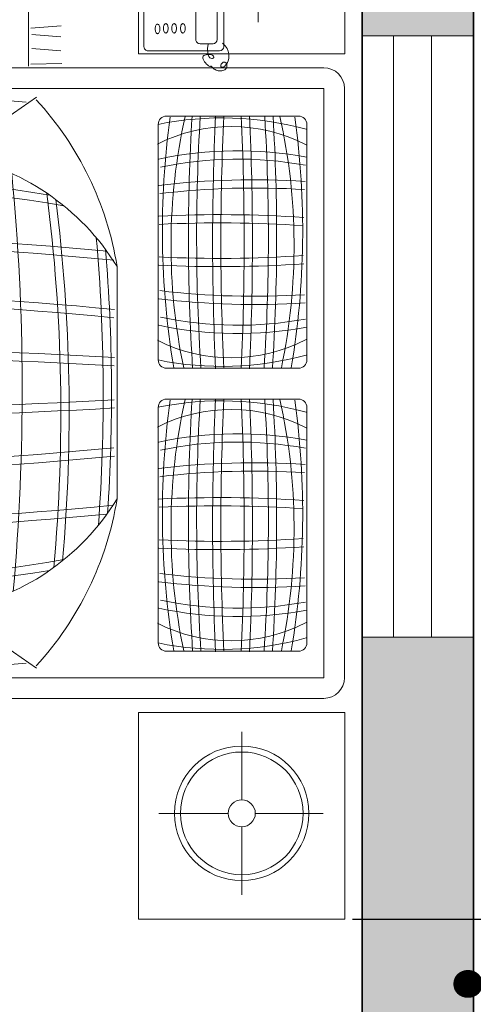
# Model space of a CAD drawing. Units: inches. Extents: x 1763 to 2368, y 1500 to 2097.
# Tile 20 of 24: x 2152 to 2189, y 1856 to 1935. Entities that reach past the tile are written whole.
import ezdxf

# ---------------------------------------------------------------- set-up
doc = ezdxf.new("R2010")
doc.units = ezdxf.units.IN
for name, color, linetype, lineweight in [('A-ANNO-DIMS', 2, 'Continuous', 18), ('A-FURN', 8, 'Continuous', 18), ('A-WALL', 7, 'Continuous', 35), ('A-WALL-PATT', 7, 'Continuous', 13), ('windows', 1, 'Continuous', 18)]:
    doc.layers.add(name, color=color, linetype=linetype, lineweight=lineweight)
doc.styles.get("Standard").update_dxf_attribs({"font": 'arial.ttf'})
doc.dimstyles.new('ISO-25', dxfattribs={"dimtxt": 12.5, "dimasz": 2.5, "dimexe": 1.25, "dimexo": 0.625, "dimtad": 1, "dimdec": 0, "dimlunit": 4, "dimtxsty": 'Standard', "dimblk": 'ARCHTICK', "dimcen": 2.5, "dimclrd": 3, "dimclrt": 4, "dimadec": 0, "dimazin": 0, "dimtfac": 1, "dimtdec": 0, "dimtmove": 0, "dimatfit": 3, "dimfxl": 1, "dimarcsym": 0})

# ---------------------------------------------------------------- blocks, each defined once
blk = doc.blocks.new('A$C77DF40FE')
for p, q in [((0.5, 2.6723), (0, 2.6723)), ((0.5, 2.1723), (0.5, 2.6723)), ((0.5839, 2.6714), (2.0097, 2.6714)), ((2.0936, 2.1723), (2.0936, 2.6723)), ((2.0936, 2.6723), (2.5936, 2.6723)), ((2.5936, 2.6723), (2.5936, 2.1723)), ((0.5339, 0.6344), (0.5339, 2.6214)), ((0.5839, 2.6214), (2.0097, 2.6214)), ((0.5839, 0.6344), (0.5839, 2.6214)), ((2.0097, 2.6214), (2.0097, 0.6344)), ((2.0597, 2.6214), (2.0597, 0.6344)), ((2.3379, 2.4554), (2.3379, 2.6199)), ((1.2408, 2.5803), (0.6708, 2.5803)), ((1.9255, 2.5803), (1.3555, 2.5803)), ((0.6508, 2.5603), (0.6508, 2.2403)), ((1.2608, 2.2403), (1.2608, 2.5603)), ((1.3355, 2.5603), (1.3355, 2.2403)), ((1.9455, 2.2403), (1.9455, 2.5603)), ((0.2588, 2.4621), (0.4233, 2.4621)), ((2.3051, 2.4226), (2.1406, 2.4226)), ((2.5352, 2.4226), (2.3707, 2.4226)), ((0.4873, 2.387), (0.4809, 2.3823)), ((0.4937, 2.3899), (0.4873, 2.387)), ((0.5, 2.3914), (0.4937, 2.3899)), ((0.506, 2.3917), (0.5, 2.3914)), ((0.5117, 2.391), (0.506, 2.3917)), ((0.5168, 2.3897), (0.5117, 2.391)), ((0.5212, 2.3878), (0.5168, 2.3897)), ((0.521, 2.3828), (0.5205, 2.3816)), ((0.5219, 2.3839), (0.521, 2.3828)), ((0.5248, 2.3858), (0.5212, 2.3878)), ((0.523, 2.3849), (0.5219, 2.3839)), ((0.5244, 2.3856), (0.523, 2.3849)), ((0.5261, 2.3861), (0.5244, 2.3856)), ((0.5277, 2.3836), (0.5248, 2.3858)), ((0.5279, 2.3864), (0.5261, 2.3861)), ((0.5298, 2.3813), (0.5277, 2.3836)), ((0.5298, 2.3864), (0.5279, 2.3864)), ((0.5318, 2.3861), (0.5298, 2.3864)), ((0.5338, 2.3855), (0.5318, 2.3861)), ((0.5356, 2.3846), (0.5338, 2.3855)), ((0.5373, 2.3832), (0.5356, 2.3846)), ((0.5387, 2.3815), (0.5373, 2.3832)), ((2.3379, 2.2215), (2.3379, 2.3898)), ((0.4828, 2.3788, 10.4), (0.2438, 2.3788, 10.4)), ((0.4656, 2.363, 10.4), (0.2638, 2.363, 10.4)), ((0.4809, 2.3823), (0.4746, 2.3757)), ((0.4928, 2.1957, 10.4), (0.4928, 2.3688, 10.4)), ((0.5205, 2.3816), (0.5202, 2.3804)), ((0.5202, 2.3804), (0.5202, 2.379)), ((0.5202, 2.379), (0.5206, 2.3777)), ((0.5206, 2.3777), (0.5213, 2.3764)), ((0.5213, 2.3764), (0.5224, 2.3752)), ((0.5224, 2.3752), (0.5237, 2.374)), ((0.5237, 2.374), (0.5252, 2.3731)), ((0.5252, 2.3731), (0.5268, 2.3723)), ((0.5268, 2.3723), (0.5283, 2.3719)), ((0.5283, 2.3719), (0.5297, 2.3717)), ((0.5297, 2.3717), (0.531, 2.372)), ((0.5313, 2.3792), (0.5298, 2.3813)), ((0.531, 2.372), (0.5319, 2.3726)), ((0.5322, 2.3771), (0.5313, 2.3792)), ((0.5319, 2.3726), (0.5325, 2.3738)), ((0.5326, 2.3753), (0.5322, 2.3771)), ((0.5325, 2.3738), (0.5326, 2.3753)), ((0.5383, 2.3581), (0.5394, 2.3604)), ((0.5399, 2.3794), (0.5387, 2.3815)), ((0.5394, 2.3604), (0.5403, 2.3629)), ((0.5407, 2.377), (0.5399, 2.3794)), ((0.5403, 2.3629), (0.5409, 2.3657)), ((0.5412, 2.3743), (0.5407, 2.377)), ((0.5409, 2.3657), (0.5413, 2.3686)), ((0.5414, 2.3715), (0.5412, 2.3743)), ((0.5413, 2.3686), (0.5414, 2.3715)), ((0.4756, 2.3215, 10.4), (0.4756, 2.353, 10.4)), ((0.4767, 2.3409), (0.4876, 2.34)), ((0.4876, 2.34), (0.4961, 2.3402)), ((0.4961, 2.3402), (0.5023, 2.3413)), ((0.502, 2.3463), (0.5017, 2.3431)), ((0.5017, 2.3431), (0.5018, 2.3398)), ((0.5018, 2.3398), (0.5023, 2.3365)), ((0.5026, 2.3491), (0.502, 2.3463)), ((0.5023, 2.3413), (0.5067, 2.3431)), ((0.5023, 2.3365), (0.5031, 2.3334)), ((0.5035, 2.3514), (0.5026, 2.3491)), ((0.5047, 2.3531), (0.5035, 2.3514)), ((0.5059, 2.3542), (0.5047, 2.3531)), ((0.5073, 2.3548), (0.5059, 2.3542)), ((0.5067, 2.3431), (0.5095, 2.3452)), ((0.5086, 2.3549), (0.5073, 2.3548)), ((0.5097, 2.3544), (0.5086, 2.3549)), ((0.5095, 2.3452), (0.511, 2.3475)), ((0.5107, 2.3534), (0.5097, 2.3544)), ((0.5113, 2.3518), (0.5107, 2.3534)), ((0.511, 2.3475), (0.5115, 2.3498)), ((0.5115, 2.3498), (0.5113, 2.3518)), ((0.5193, 2.3325), (0.5222, 2.3349)), ((0.5222, 2.3349), (0.5249, 2.3374)), ((0.5249, 2.3374), (0.5271, 2.3398)), ((0.5271, 2.3398), (0.5288, 2.3419)), ((0.5288, 2.3419), (0.5299, 2.3436)), ((0.5299, 2.3436), (0.5305, 2.3449)), ((0.53, 2.3482), (0.5302, 2.3488)), ((0.5301, 2.3477), (0.53, 2.3482)), ((0.5303, 2.3472), (0.5301, 2.3477)), ((0.5302, 2.3488), (0.5308, 2.3495)), ((0.5306, 2.3466), (0.5303, 2.3472)), ((0.5305, 2.3449), (0.5307, 2.3459)), ((0.5307, 2.3459), (0.5306, 2.3466)), ((0.5308, 2.3495), (0.5317, 2.3504)), ((0.5317, 2.3504), (0.5329, 2.3515)), ((0.5329, 2.3515), (0.5342, 2.3528)), ((0.5342, 2.3528), (0.5356, 2.3543)), ((0.5356, 2.3543), (0.537, 2.3561)), ((0.537, 2.3561), (0.5383, 2.3581)), ((0.2638, 2.3115, 10.4), (0.4656, 2.3115, 10.4)), ((0.5031, 2.3334), (0.5043, 2.3309)), ((0.5043, 2.3309), (0.506, 2.329)), ((0.506, 2.329), (0.5081, 2.328)), ((0.5081, 2.328), (0.5106, 2.328)), ((0.5106, 2.328), (0.5134, 2.3288)), ((0.5134, 2.3288), (0.5163, 2.3304)), ((0.5163, 2.3304), (0.5193, 2.3325)), ((0.6708, 2.2203), (1.2408, 2.2203)), ((1.3555, 2.2203), (1.9255, 2.2203)), ((0, 2.1723), (0.5, 2.1723)), ((0.2438, 2.1857, 10.4), (0.4828, 2.1857, 10.4)), ((2.5936, 2.1723), (2.0936, 2.1723)), ((1.5773, 2.1205), (1.0147, 2.1205)), ((0.438, 1.9118), (0.4323, 1.9849)), ((0.4531, 1.9138), (0.4588, 1.9847)), ((0.4873, 1.9138), (0.493, 1.9847)), ((0.5249, 1.9118), (0.5233, 1.9865)), ((0.6051, 1.925), (0.7457, 1.7234)), ((1.9869, 1.925), (1.8463, 1.7234)), ((0.5301, 1.9057), (0.3112, 1.9057))]:
    blk.add_line(p, q)
for radius in [0.1629, 0.1484, 0.0328]:
    blk.add_circle((2.3379, 2.4226), radius)
for centre, radius, start, end in [((0.5839, 2.6214), 0.05, 90, 180), ((2.0097, 2.6214), 0.05, 0, 90), ((0.6708, 2.5603), 0.02, 90, 180), ((1.4247, 2.3742), 0.7696, 164.6112, 191.5679), ((1.0701, 2.3966), 0.3942, 152.5365, 206.92), ((1.6628, 2.4129), 0.928, 169.6087, 191.899), ((1.6628, 2.4129), 0.908, 169.6087, 191.899), ((2.7571, 2.4533), 1.9523, 176.3947, 186.8195), ((2.7571, 2.4533), 1.9323, 176.3947, 186.8195), ((-0.8455, 2.4533), 1.9323, 353.1805, 3.6053), ((-0.8455, 2.4533), 1.9523, 353.1805, 3.6053), ((0.2489, 2.4129), 0.908, 348.101, 10.3913), ((0.2489, 2.4129), 0.928, 348.101, 10.3913), ((0.8416, 2.3966), 0.3942, 333.08, 27.4635), ((0.4869, 2.3742), 0.7696, 348.4321, 15.3888), ((1.2408, 2.5603), 0.02, 0, 90), ((1.3555, 2.5603), 0.02, 90, 180), ((2.1094, 2.3742), 0.7696, 164.6112, 191.5679), ((1.7548, 2.3966), 0.3942, 152.5365, 206.92), ((2.3475, 2.4129), 0.928, 169.6087, 191.899), ((2.3475, 2.4129), 0.908, 169.6087, 191.899), ((3.4419, 2.4533), 1.9523, 176.3947, 186.8195), ((3.4419, 2.4533), 1.9323, 176.3947, 186.8195), ((-0.1608, 2.4533), 1.9323, 353.1805, 3.6053), ((-0.1608, 2.4533), 1.9523, 353.1805, 3.6053), ((0.9336, 2.4129), 0.908, 348.101, 10.3913), ((0.9336, 2.4129), 0.928, 348.101, 10.3913), ((1.5263, 2.3966), 0.3942, 333.08, 27.4635), ((1.1716, 2.3742), 0.7696, 348.4321, 15.3888), ((1.9255, 2.5603), 0.02, 0, 90), ((0.9635, 1.1066), 1.4427, 78.1527, 102.4906), ((0.9287, 0.5819), 1.9884, 80.4201, 97.9672), ((3.9259, 2.3685), 3.0367, 176.1432, 182.775), ((3.9259, 2.3685), 3.0167, 176.1432, 182.775), ((-2.0216, 2.3685), 3.0167, 357.225, 3.8568), ((-2.0216, 2.3685), 3.0367, 357.225, 3.8568), ((1.6482, 1.1066), 1.4427, 78.1527, 102.4906), ((1.6135, 0.5819), 1.9884, 80.4201, 97.9672), ((4.6106, 2.3685), 3.0367, 176.1432, 182.775), ((4.6106, 2.3685), 3.0167, 176.1432, 182.775), ((-1.3369, 2.3685), 3.0167, 357.225, 3.8568), ((-1.3369, 2.3685), 3.0367, 357.225, 3.8568), ((0.9445, -2.3575), 4.8647, 86.2671, 93.4563), ((1.6292, -2.3575), 4.8647, 86.2671, 93.4563), ((0.9445, -2.3575), 4.8447, 86.2671, 93.4563), ((1.6292, -2.3575), 4.8447, 86.2671, 93.4563), ((0.9561, -3.928), 6.3765, 87.24779, 92.75221), ((1.6408, -3.928), 6.3765, 87.24779, 92.75221), ((0.9561, -3.928), 6.3565, 87.24779, 92.75221), ((1.6408, -3.928), 6.3565, 87.24779, 92.75221), ((0.4656, 2.353, 10.4), 0.01, 0, 90), ((0.4828, 2.3688, 10.4), 0.01, 0, 90), ((0.9561, 8.7285), 6.3765, 267.24779, 272.75221), ((0.9561, 8.7285), 6.3565, 267.24779, 272.75221), ((1.6408, 8.7285), 6.3765, 267.24779, 272.75221), ((1.6408, 8.7285), 6.3565, 267.24779, 272.75221), ((0.4656, 2.3215, 10.4), 0.01, 270, 0), ((0.9445, 7.158), 4.8447, 266.5437, 273.7329), ((1.6292, 7.158), 4.8447, 266.5437, 273.7329), ((0.9445, 7.158), 4.8647, 266.5437, 273.7329), ((1.6292, 7.158), 4.8647, 266.5437, 273.7329), ((0.43, 2.2801, 10.4), 0.00304, 140.3607, 180), ((0.43, 2.2801, 10.4), 0.00304, 180, 219.6393), ((0.434, 2.2768, 10.4), 0.00822, 116.5651, 140.3607), ((0.434, 2.2834, 10.4), 0.00822, 219.6393, 243.4349), ((0.4367, 2.2714, 10.4), 0.0142, 101.7009, 116.5651), ((0.4367, 2.2887, 10.4), 0.0142, 243.4349, 258.2991), ((0.4367, 2.25, 10.4), 0.0142, 101.7009, 116.5651), ((0.4384, 2.263, 10.4), 0.0228, 90, 101.7009), ((0.4384, 2.2972, 10.4), 0.0228, 258.2991, 270), ((0.4384, 2.2415, 10.4), 0.0228, 90, 101.7009), ((0.4384, 2.263, 10.4), 0.0228, 78.2991, 90), ((0.4384, 2.2972, 10.4), 0.0228, 270, 281.7009), ((0.4384, 2.2415, 10.4), 0.0228, 78.2991, 90), ((0.4402, 2.2714, 10.4), 0.0142, 63.4349, 78.2991), ((0.4402, 2.2887, 10.4), 0.0142, 281.7009, 296.5651), ((0.4402, 2.25, 10.4), 0.0142, 63.4349, 78.2991), ((0.4428, 2.2768, 10.4), 0.00822, 39.6393, 63.4349), ((0.4428, 2.2834, 10.4), 0.00822, 296.5651, 320.3607), ((0.4468, 2.2801, 10.4), 0.00304, 0, 39.6393), ((0.4468, 2.2801, 10.4), 0.00304, 320.3607, 0), ((0.9635, 3.6939), 1.4427, 257.5094, 281.8473), ((1.6482, 3.6939), 1.4427, 257.5094, 281.8473), ((0.43, 2.2586, 10.4), 0.00304, 140.3607, 180), ((0.43, 2.2586, 10.4), 0.00304, 180, 219.6393), ((0.43, 2.2386, 10.4), 0.00304, 140.3607, 180), ((0.434, 2.2553, 10.4), 0.00822, 116.5651, 140.3607), ((0.434, 2.2619, 10.4), 0.00822, 219.6393, 243.4349), ((0.434, 2.2353, 10.4), 0.00822, 116.5651, 140.3607), ((0.4367, 2.2673, 10.4), 0.0142, 243.4349, 258.2991), ((0.4367, 2.23, 10.4), 0.0142, 101.7009, 116.5651), ((0.4384, 2.2757, 10.4), 0.0228, 258.2991, 270), ((0.4384, 2.2215, 10.4), 0.0228, 90, 101.7009), ((0.4384, 2.2757, 10.4), 0.0228, 270, 281.7009), ((0.4384, 2.2215, 10.4), 0.0228, 78.2991, 90), ((0.4402, 2.2673, 10.4), 0.0142, 281.7009, 296.5651), ((0.4402, 2.23, 10.4), 0.0142, 63.4349, 78.2991), ((0.4428, 2.2553, 10.4), 0.00822, 39.6393, 63.4349), ((0.4428, 2.2619, 10.4), 0.00822, 296.5651, 320.3607), ((0.4428, 2.2353, 10.4), 0.00822, 39.6393, 63.4349), ((0.4468, 2.2586, 10.4), 0.00304, 0, 39.6393), ((0.4468, 2.2586, 10.4), 0.00304, 320.3607, 0), ((0.4468, 2.2386, 10.4), 0.00304, 0, 39.6393), ((0.6708, 2.2403), 0.02, 180, 270), ((0.9287, 4.2186), 1.9884, 262.0328, 279.5799), ((1.2408, 2.2403), 0.02, 270, 0), ((1.3555, 2.2403), 0.02, 180, 270), ((1.6135, 4.2186), 1.9884, 262.0328, 279.5799), ((1.9255, 2.2403), 0.02, 270, 0), ((0.43, 2.2386, 10.4), 0.00304, 180, 219.6393), ((0.434, 2.2419, 10.4), 0.00822, 219.6393, 243.4349), ((0.4314, 2.2186, 10.4), 0.00304, 140.3607, 180), ((0.4314, 2.2186, 10.4), 0.00304, 180, 219.6393), ((0.4354, 2.2153, 10.4), 0.00822, 116.5651, 140.3607), ((0.4354, 2.2219, 10.4), 0.00822, 219.6393, 243.4349), ((0.4367, 2.2472, 10.4), 0.0142, 243.4349, 258.2991), ((0.4381, 2.2099, 10.4), 0.0142, 101.7009, 116.5651), ((0.4384, 2.2557, 10.4), 0.0228, 258.2991, 270), ((0.4398, 2.2015, 10.4), 0.0228, 90, 101.7009), ((0.4384, 2.2557, 10.4), 0.0228, 270, 281.7009), ((0.4398, 2.2015, 10.4), 0.0228, 78.2991, 90), ((0.4402, 2.2472, 10.4), 0.0142, 281.7009, 296.5651), ((0.4416, 2.2099, 10.4), 0.0142, 63.4349, 78.2991), ((0.4428, 2.2419, 10.4), 0.00822, 296.5651, 320.3607), ((0.4443, 2.2153, 10.4), 0.00822, 39.6393, 63.4349), ((0.4443, 2.2219, 10.4), 0.00822, 296.5651, 320.3607), ((0.4468, 2.2386, 10.4), 0.00304, 320.3607, 0), ((0.4483, 2.2186, 10.4), 0.00304, 0, 39.6393), ((0.4483, 2.2186, 10.4), 0.00304, 320.3607, 0), ((0.4381, 2.2272, 10.4), 0.0142, 243.4349, 258.2991), ((0.4398, 2.2357, 10.4), 0.0228, 258.2991, 270), ((0.4398, 2.2357, 10.4), 0.0228, 270, 281.7009), ((0.4416, 2.2272, 10.4), 0.0142, 281.7009, 296.5651), ((0.4828, 2.1957, 10.4), 0.01, 270, 0), ((1.1396, 1.3485), 0.782, 99.1908, 132.5116), ((1.3217, 1.6229), 0.5847, 121.6676, 170.1065), ((1.2703, 1.6229), 0.5847, 9.8935, 58.3324), ((1.4523, 1.3485), 0.782, 47.4884, 80.8092), ((10.1174, 1.2237), 9.161, 174.43278, 183.67204), ((1.3248, -2.1722), 4.2793, 86.1532, 94.7091), ((10.2564, 1.2237), 9.181, 174.43278, 183.67204), ((10.2564, 1.2237), 9.161, 174.43278, 183.67204), ((16.3019, 1.253), 15.0916, 176.72768, 182.32074), ((16.3019, 1.253), 15.0716, 176.72768, 182.32074), ((-13.7099, 1.253), 15.0716, 357.67926, 3.27232), ((-13.7099, 1.253), 15.0916, 357.67926, 3.27232), ((-7.6644, 1.2237), 9.161, 356.32796, 5.56722), ((-7.6644, 1.2237), 9.181, 356.32796, 5.56722), ((-7.5254, 1.2237), 9.161, 356.32796, 5.55658), ((10.1174, 1.2237), 9.181, 174.54912, 183.67204), ((1.3248, -2.1722), 4.2593, 85.7473, 95.1159), ((-7.5254, 1.2237), 9.181, 356.32796, 5.45088), ((1.3657, -2.1044), 4.1088, 84.9619, 97.1707), ((4.947, 1.2796), 4.1406, 170.0939, 188.8179), ((1.3657, -2.1044), 4.0888, 84.7053, 97.4283), ((-2.355, 1.2796), 4.1406, 351.1821, 9.9061), ((4.947, 1.2796), 4.1606, 170.6272, 188.8179), ((-2.355, 1.2796), 4.1606, 351.1821, 9.3728), ((7.8077, 1.3061), 7.2149, 175.27403, 185.28261), ((1.3142, -3.5764), 5.4671, 84.8953, 95.5052), ((-5.2157, 1.3061), 7.2149, 354.71739, 4.72597)]:
    blk.add_arc(centre, radius, start, end)
blk = doc.blocks.new('_ArchTick')
at = {"color": 0, "linetype": 'ByBlock', "const_width": 0.15}
blk.add_lwpolyline([(-0.5, -0.5), (0.5, 0.5)], dxfattribs=at)
blk = doc.blocks.new('*D22')
at = {"layer": 'A-ANNO-DIMS', "color": 0, "lineweight": -2, "transparency": 16777216}
for p, q in [((2189.717, 2043.273), (2269.316, 2043.273)), ((2268.066, 2043.273), (2268.066, 1563.273)), ((2189.717, 1563.273), (2269.316, 1563.273))]:
    blk.add_line(p, q, dxfattribs=at)
at = {"layer": 'Defpoints', "color": 0, "transparency": 16777216}
for p in [(2189.092, 2043.273), (2189.092, 1563.273), (2268.066, 1563.273)]:
    blk.add_point(p, dxfattribs=at)
at = {"layer": 'A-ANNO-DIMS', "color": 0, "lineweight": -2, "transparency": 16777216, "xscale": 2.5, "yscale": 2.5, "zscale": 2.5}
for p, rotation in [((2268.066, 2043.273), 90), ((2268.066, 1563.273), 270)]:
    blk.add_blockref('_ArchTick', p, dxfattribs=dict(at, rotation=rotation))
at = {"layer": 'A-ANNO-DIMS', "color": 0, "transparency": 16777216, "insert": (2261.059, 1803.273), "char_height": 12.5, "attachment_point": 5, "rotation": 90}
blk.add_mtext("40'", dxfattribs=at)
blk = doc.blocks.new('*D23')
at = {"layer": 'A-ANNO-DIMS', "color": 0, "lineweight": -2, "transparency": 16777216}
for p, q in [((2089.477, 1949.977), (2089.477, 1963.985)), ((2178.698, 1949.977), (2178.698, 1963.985))]:
    blk.add_line(p, q, dxfattribs=at)
at = {"layer": 'A-ANNO-DIMS', "color": 3, "lineweight": -2, "transparency": 16777216}
for p, q in [((2089.477, 1962.735), (2178.698, 1962.735)), ((2178.698, 1962.735), (2367.732, 1962.735))]:
    blk.add_line(p, q, dxfattribs=at)
at = {"layer": 'Defpoints', "color": 0, "transparency": 16777216}
for p in [(2178.698, 1962.735), (2089.477, 1949.352), (2178.698, 1949.352)]:
    blk.add_point(p, dxfattribs=at)
at = {"layer": 'A-ANNO-DIMS', "color": 3, "lineweight": -2, "transparency": 16777216, "xscale": 2.5, "yscale": 2.5, "zscale": 2.5, "rotation": 180}
blk.add_blockref('_ArchTick', (2089.477, 1962.735), dxfattribs=at)
at = {"layer": 'A-ANNO-DIMS', "color": 3, "lineweight": -2, "transparency": 16777216, "xscale": 2.5, "yscale": 2.5, "zscale": 2.5}
blk.add_blockref('_ArchTick', (2178.698, 1962.735), dxfattribs=at)
at = {"layer": 'A-ANNO-DIMS', "color": 4, "transparency": 16777216, "insert": (2274.465, 1969.828), "char_height": 12.5, "attachment_point": 5}
blk.add_mtext('BED GROUP 7\'-5" TYP.', dxfattribs=at)
blk = doc.blocks.new('*D24')
at = {"layer": 'A-ANNO-DIMS', "color": 0, "lineweight": -2, "transparency": 16777216}
for p, q in [((2179.323, 1949.352), (2193.332, 1949.352)), ((2179.323, 1862.758), (2193.332, 1862.758))]:
    blk.add_line(p, q, dxfattribs=at)
at = {"layer": 'A-ANNO-DIMS', "color": 3, "lineweight": -2, "transparency": 16777216}
for p, q in [((2192.082, 1949.352), (2192.082, 1862.758)), ((2192.082, 1862.758), (2192.082, 1753.79))]:
    blk.add_line(p, q, dxfattribs=at)
at = {"layer": 'Defpoints', "color": 0, "transparency": 16777216}
for p in [(2178.698, 1949.352), (2178.698, 1862.758), (2192.082, 1862.758)]:
    blk.add_point(p, dxfattribs=at)
at = {"layer": 'A-ANNO-DIMS', "color": 3, "lineweight": -2, "transparency": 16777216, "xscale": 2.5, "yscale": 2.5, "zscale": 2.5}
for p, rotation in [((2192.082, 1949.352), 90), ((2192.082, 1862.758), 270)]:
    blk.add_blockref('_ArchTick', p, dxfattribs=dict(at, rotation=rotation))
at = {"layer": 'A-ANNO-DIMS', "color": 4, "transparency": 16777216, "insert": (2184.993, 1807.024), "char_height": 12.5, "attachment_point": 5, "rotation": 90}
blk.add_mtext('7\'-2 1/2" TYP.', dxfattribs=at)
blk = doc.blocks.new('*D62')
at = {"layer": 'A-ANNO-DIMS', "color": 0, "lineweight": -2, "transparency": 16777216}
for p, q in [((2083.092, 1980.648), (2083.092, 1509.906)), ((2120.612, 1980.648), (2120.612, 1509.906))]:
    blk.add_line(p, q, dxfattribs=at)
at = {"layer": 'A-ANNO-DIMS', "color": 3, "lineweight": -2, "transparency": 16777216}
for p, q in [((2083.092, 1511.156), (2120.612, 1511.156)), ((2120.612, 1511.156), (2186.709, 1511.156))]:
    blk.add_line(p, q, dxfattribs=at)
at = {"layer": 'Defpoints', "color": 0, "transparency": 16777216}
for p in [(2083.092, 1981.273), (2120.612, 1981.273), (2120.612, 1511.156)]:
    blk.add_point(p, dxfattribs=at)
at = {"layer": 'A-ANNO-DIMS', "color": 3, "lineweight": -2, "transparency": 16777216, "xscale": 2.5, "yscale": 2.5, "zscale": 2.5, "rotation": 180}
blk.add_blockref('_ArchTick', (2083.092, 1511.156), dxfattribs=at)
at = {"layer": 'A-ANNO-DIMS', "color": 3, "lineweight": -2, "transparency": 16777216, "xscale": 2.5, "yscale": 2.5, "zscale": 2.5}
blk.add_blockref('_ArchTick', (2120.612, 1511.156), dxfattribs=at)
at = {"layer": 'A-ANNO-DIMS', "color": 4, "transparency": 16777216, "insert": (2154.91, 1518.249), "char_height": 12.5, "attachment_point": 5}
blk.add_mtext('3\'-1 1/2"', dxfattribs=at)
blk = doc.blocks.new('*D78')
at = {"layer": 'A-ANNO-DIMS', "color": 0, "lineweight": -2, "transparency": 16777216}
for p, q in [((1996.717, 1981.273), (2217.842, 1981.273)), ((1986.217, 1948.273), (2217.842, 1948.273))]:
    blk.add_line(p, q, dxfattribs=at)
at = {"layer": 'A-ANNO-DIMS', "color": 3, "lineweight": -2, "transparency": 16777216}
for p, q in [((2216.592, 1981.273), (2216.592, 1948.273)), ((2216.592, 1948.273), (2216.592, 1911.081))]:
    blk.add_line(p, q, dxfattribs=at)
at = {"layer": 'Defpoints', "color": 0, "transparency": 16777216}
for p in [(1996.092, 1981.273), (1985.592, 1948.273), (2216.592, 1948.273)]:
    blk.add_point(p, dxfattribs=at)
at = {"layer": 'A-ANNO-DIMS', "color": 3, "lineweight": -2, "transparency": 16777216, "xscale": 2.5, "yscale": 2.5, "zscale": 2.5}
for p, rotation in [((2216.592, 1981.273), 90), ((2216.592, 1948.273), 270)]:
    blk.add_blockref('_ArchTick', p, dxfattribs=dict(at, rotation=rotation))
at = {"layer": 'A-ANNO-DIMS', "color": 4, "transparency": 16777216, "insert": (2209.585, 1928.427), "char_height": 12.5, "attachment_point": 5, "rotation": 90}
blk.add_mtext('2\'-9"', dxfattribs=at)
blk = doc.blocks.new('*D95')
at = {"layer": 'A-ANNO-DIMS', "color": 0, "lineweight": -2, "transparency": 16777216}
for p, q in [((2125.159, 1998.768), (2217.842, 1998.768)), ((2121.237, 1986.273), (2217.842, 1986.273))]:
    blk.add_line(p, q, dxfattribs=at)
at = {"layer": 'A-ANNO-DIMS', "color": 3, "lineweight": -2, "transparency": 16777216}
for p, q in [((2216.592, 1998.768), (2216.592, 1986.273)), ((2216.592, 1986.273), (2216.592, 1921.344))]:
    blk.add_line(p, q, dxfattribs=at)
at = {"layer": 'Defpoints', "color": 0, "transparency": 16777216}
for p in [(2124.534, 1998.768), (2120.612, 1986.273), (2216.592, 1986.273)]:
    blk.add_point(p, dxfattribs=at)
at = {"layer": 'A-ANNO-DIMS', "color": 3, "lineweight": -2, "transparency": 16777216, "xscale": 2.5, "yscale": 2.5, "zscale": 2.5}
for p, rotation in [((2216.592, 1998.768), 90), ((2216.592, 1986.273), 270)]:
    blk.add_blockref('_ArchTick', p, dxfattribs=dict(at, rotation=rotation))
at = {"layer": 'A-ANNO-DIMS', "color": 4, "transparency": 16777216, "insert": (2209.504, 1952.559), "char_height": 12.5, "attachment_point": 5, "rotation": 90}
blk.add_mtext('1\'-0 1/2"', dxfattribs=at)

msp = doc.modelspace()

# ---------------------------------------------------------------- hatches: boundary and pattern name
at = {"layer": 'A-WALL-PATT'}
h = msp.add_hatch(color=256, dxfattribs=at)
h.dxf.hatch_style = 1
h.paths.add_polyline_path([(1838.092, 2034.273), (1838.092, 2043.273), (1829.092, 2043.273), (1829.092, 1953.387), (1838.092, 1953.387)])
h.paths.add_polyline_path([(1838.092, 1913.101), (1829.092, 1913.101), (1829.092, 1862.202), (1838.092, 1862.202)])
h.paths.add_polyline_path([(1838.092, 1825.59), (1829.092, 1825.59), (1829.092, 1738.643), (1838.092, 1738.643)])
h.paths.add_polyline_path([(1895.592, 1885.273), (1838.092, 1885.273), (1838.092, 1880.273), (1895.592, 1880.273)])
h.paths.add_polyline_path([(1857.389, 1784.273), (1838.092, 1784.273), (1838.092, 1779.273), (1857.389, 1779.273)])
h.paths.add_polyline_path([(1958.092, 1981.273), (1971.455, 1981.273), (1971.455, 1986.273), (1968.568, 1986.273), (1958.092, 1986.273), (1953.092, 1986.273), (1927.39, 1986.273), (1927.39, 1981.273), (1953.092, 1981.273), (1953.092, 1885.273), (1932.014, 1885.273), (1932.014, 1880.273), (1959.134, 1880.273), (1959.134, 1883.738), (1959.134, 1885.273), (1958.092, 1885.273)])
h.paths.add_polyline_path([(2018.092, 1981.273), (2031.019, 1981.273), (2031.019, 1986.273), (2018.092, 1986.273), (2013.092, 1986.273), (2001.233, 1986.273), (2001.233, 1981.273), (2013.092, 1981.273), (2013.092, 1885.273), (1982.182, 1885.273, -0.016629), (1982.233, 1883.738), (1982.233, 1880.273), (2049.686, 1880.273), (2049.686, 1883.738, -0.016629), (2049.737, 1885.273), (2018.092, 1885.273)])
h.paths.add_polyline_path([(2083.092, 1981.273), (2120.612, 1981.273), (2120.612, 1986.273), (2083.092, 1986.273), (2078.092, 1986.273), (2063.143, 1986.273), (2063.143, 1981.273), (2078.092, 1981.273), (2078.092, 1885.273), (2072.785, 1885.273), (2072.785, 1883.738), (2072.785, 1880.273), (2078.092, 1880.273), (2078.092, 1866.867), (2081.557, 1866.867, -0.016629), (2083.092, 1866.816)])
h.paths.add_polyline_path([(1871.675, 1635.273), (1838.092, 1635.273), (1838.092, 1626.273), (1871.675, 1626.273)], flags=17)
h.paths.add_polyline_path([(2100.577, 1688.273), (2060.092, 1688.273), (2060.092, 1679.273), (2100.577, 1679.273)], flags=17)
h.paths.add_polyline_path([(2180.092, 1688.273), (2148.744, 1688.273), (2148.744, 1679.273), (2180.092, 1679.273)], flags=17)
h.paths.add_polyline_path([(2189.092, 1746.219), (2180.092, 1746.219), (2180.092, 1743.417), (2180.123, 1743.417), (2180.123, 1726.723), (2180.092, 1572.273), (2034.907, 1572.273), (2034.907, 1565.601), (2034.907, 1563.273), (2189.092, 1563.273)])
h.paths.add_polyline_path([(2060.092, 1802.347, -0.016629), (2058.557, 1802.296), (2055.092, 1802.296), (2055.092, 1635.273), (2042.484, 1635.273), (2042.484, 1629.738), (2042.484, 1626.273), (2055.092, 1626.273), (2055.092, 1599.273), (2040.269, 1599.273), (2040.269, 1590.273), (2060.092, 1590.273)])
h.paths.add_polyline_path([(2019.385, 1629.738, -0.060569), (2020.058, 1635.273), (1995.092, 1635.273), (1990.092, 1635.273), (1927.075, 1635.273), (1927.075, 1626.273), (1990.092, 1626.273), (1990.092, 1590.273), (1995.092, 1590.273), (2005.195, 1590.273), (2005.195, 1599.273), (1995.092, 1599.273), (1995.092, 1626.273), (2019.385, 1626.273)])
edge = h.paths.add_edge_path()
edge.add_line((2180.092, 1837.273), (2167.198, 1837.273))
edge.add_spline(control_points=[(2167.198, 1837.273), (2167.191, 1837.271), (2167.183, 1837.271), (2167.176, 1837.273)], knot_values=[168.955493, 168.955493, 168.955493, 168.955493, 169.065871, 169.065871, 169.065871, 169.065871], degree=3, periodic=0)
edge.add_spline(control_points=[(2167.176, 1837.273), (2166.556, 1837.377), (2166.326, 1846.161), (2165.708, 1846.244)], knot_values=[159.864705, 159.864705, 159.864705, 159.864705, 168.955493, 168.955493, 168.955493, 168.955493], degree=3, periodic=0)
edge.add_line((2167.122, 1837.273), (2163.16, 1837.273))
edge.add_spline(control_points=[(2163.16, 1837.273), (2163.158, 1837.273), (2163.156, 1837.273), (2163.155, 1837.273)], knot_values=[150.537172, 150.537172, 150.537172, 150.537172, 150.553797, 150.553797, 150.553797, 150.553797], degree=3, periodic=0)
edge.add_spline(control_points=[(2163.155, 1837.273), (2162.29, 1837.289), (2161.594, 1846.232), (2160.878, 1846.244)], knot_values=[141.293426, 141.293426, 141.293426, 141.293426, 150.537172, 150.537172, 150.537172, 150.537172], degree=3, periodic=0)
edge.add_line((2163.075, 1837.273), (2158.7, 1837.273))
edge.add_spline(control_points=[(2158.7, 1837.273), (2158.698, 1837.273), (2158.697, 1837.273), (2158.696, 1837.273)], knot_values=[132.033544, 132.033544, 132.033544, 132.033544, 132.049151, 132.049151, 132.049151, 132.049151], degree=3, periodic=0)
edge.add_spline(control_points=[(2158.696, 1837.273), (2157.972, 1837.288), (2157.262, 1846.233), (2156.393, 1846.244)], knot_values=[122.786021, 122.786021, 122.786021, 122.786021, 132.033544, 132.033544, 132.033544, 132.033544], degree=3, periodic=0)
edge.add_line((2158.629, 1837.273), (2153.839, 1837.273))
edge.add_spline(control_points=[(2153.839, 1837.273), (2153.831, 1837.271), (2153.823, 1837.271), (2153.816, 1837.273)], knot_values=[113.451585, 113.451585, 113.451585, 113.451585, 113.562103, 113.562103, 113.562103, 113.562103], degree=3, periodic=0)
edge.add_spline(control_points=[(2153.816, 1837.273), (2153.17, 1837.378), (2152.878, 1846.191), (2152.404, 1846.244)], knot_values=[0, 0, 0, 0, 9.081854, 9.081854, 9.081854, 9.081854], degree=3, periodic=0)
edge.add_line((2153.76, 1837.273), (2150.391, 1837.273))
edge.add_spline(control_points=[(2150.391, 1837.273), (2150.381, 1837.272), (2150.371, 1837.272), (2150.361, 1837.273)], knot_values=[95.069382, 95.069382, 95.069382, 95.069382, 95.17519, 95.17519, 95.17519, 95.17519], degree=3, periodic=0)
edge.add_spline(control_points=[(2150.361, 1837.273), (2149.487, 1837.373), (2148.419, 1846.194), (2147.589, 1846.244)], knot_values=[85.824599, 85.824599, 85.824599, 85.824599, 95.069382, 95.069382, 95.069382, 95.069382], degree=3, periodic=0)
edge.add_line((2150.286, 1837.273), (2145.43, 1837.273))
edge.add_spline(control_points=[(2145.43, 1837.273), (2145.426, 1837.273), (2145.423, 1837.273), (2145.419, 1837.273)], knot_values=[76.505559, 76.505559, 76.505559, 76.505559, 76.547811, 76.547811, 76.547811, 76.547811], degree=3, periodic=0)
edge.add_spline(control_points=[(2145.419, 1837.273), (2144.684, 1837.313), (2143.804, 1846.194), (2142.948, 1846.244)], knot_values=[67.23945, 67.23945, 67.23945, 67.23945, 76.505559, 76.505559, 76.505559, 76.505559], degree=3, periodic=0)
edge.add_line((2145.353, 1837.273), (2134.57, 1837.273))
edge.add_spline(control_points=[(2134.57, 1837.273), (2134.567, 1837.272), (2134.563, 1837.272), (2134.56, 1837.273)], knot_values=[39.001463, 39.001463, 39.001463, 39.001463, 39.045107, 39.045107, 39.045107, 39.045107], degree=3, periodic=0)
edge.add_spline(control_points=[(2134.56, 1837.273), (2133.872, 1837.313), (2133.397, 1845.853), (2132.328, 1846.244)], knot_values=[29.79778, 29.79778, 29.79778, 29.79778, 39.001463, 39.001463, 39.001463, 39.001463], degree=3, periodic=0)
edge.add_line((2134.498, 1837.273), (2128.075, 1837.273))
edge.add_spline(control_points=[(2128.075, 1837.273), (2128.026, 1837.26), (2127.978, 1837.26), (2127.931, 1837.273)], knot_values=[19.482067, 19.482067, 19.482067, 19.482067, 19.869396, 19.869396, 19.869396, 19.869396], degree=3, periodic=0)
edge.add_spline(control_points=[(2125.013, 1846.244), (2126.165, 1844.663), (2126.821, 1837.57), (2127.931, 1837.273)], knot_values=[10.389805, 10.389805, 10.389805, 10.389805, 19.482067, 19.482067, 19.482067, 19.482067], degree=3, periodic=0)
edge.add_line((2127.931, 1837.273), (2083.092, 1837.273))
edge.add_line((2083.092, 1837.273), (2083.092, 1843.768))
edge.add_line((2083.092, 1843.768), (2081.557, 1843.768))
edge.add_line((2081.557, 1843.768), (2078.092, 1843.768))
edge.add_line((2078.092, 1843.768), (2078.092, 1837.273))
edge.add_line((2078.092, 1837.273), (2055.092, 1837.273))
edge.add_line((2055.092, 1837.273), (2055.092, 1825.395))
edge.add_line((2055.092, 1825.395), (2058.557, 1825.395))
edge.add_line((2058.557, 1825.395), (2060.092, 1825.395))
edge.add_line((2060.092, 1825.395), (2060.092, 1832.273))
edge.add_line((2060.092, 1832.273), (2122.437, 1832.273))
edge.add_spline(control_points=[(2122.437, 1832.273), (2122.727, 1832.584), (2123.008, 1832.617), (2123.275, 1832.273)], knot_values=[5.972033, 5.972033, 5.972033, 5.972033, 8.057258, 8.057258, 8.057258, 8.057258], degree=3, periodic=0)
edge.add_line((2123.275, 1832.273), (2137.951, 1832.273))
edge.add_spline(control_points=[(2137.951, 1832.273), (2137.961, 1832.274), (2137.971, 1832.274), (2137.98, 1832.273)], knot_values=[53.926862, 53.926862, 53.926862, 53.926862, 54.030075, 54.030075, 54.030075, 54.030075], degree=3, periodic=0)
edge.add_spline(control_points=[(2139.716, 1825.016), (2139.281, 1825.062), (2138.671, 1832.176), (2137.98, 1832.273)], knot_values=[54.030075, 54.030075, 54.030075, 54.030075, 61.445194, 61.445194, 61.445194, 61.445194], degree=3, periodic=0)
edge.add_line((2138.045, 1832.273), (2140.962, 1832.273))
edge.add_spline(control_points=[(2140.962, 1832.273), (2140.971, 1832.274), (2140.98, 1832.274), (2140.988, 1832.273)], knot_values=[68.854182, 68.854182, 68.854182, 68.854182, 68.971237, 68.971237, 68.971237, 68.971237], degree=3, periodic=0)
edge.add_spline(control_points=[(2143.19, 1825.016), (2142.436, 1825.065), (2141.561, 1832.162), (2140.988, 1832.273)], knot_values=[68.971237, 68.971237, 68.971237, 68.971237, 76.444911, 76.444911, 76.444911, 76.444911], degree=3, periodic=0)
edge.add_line((2141.041, 1832.273), (2145.43, 1832.273))
edge.add_spline(control_points=[(2145.43, 1832.273), (2145.439, 1832.274), (2145.448, 1832.274), (2145.458, 1832.273)], knot_values=[84.039047, 84.039047, 84.039047, 84.039047, 84.124041, 84.124041, 84.124041, 84.124041], degree=3, periodic=0)
edge.add_spline(control_points=[(2148.108, 1825.016), (2147.34, 1825.02), (2146.303, 1832.193), (2145.458, 1832.273)], knot_values=[84.124041, 84.124041, 84.124041, 84.124041, 91.773891, 91.773891, 91.773891, 91.773891], degree=3, periodic=0)
edge.add_line((2145.538, 1832.273), (2150.393, 1832.273))
edge.add_spline(control_points=[(2150.393, 1832.273), (2150.419, 1832.277), (2150.445, 1832.277), (2150.472, 1832.273)], knot_values=[99.381577, 99.381577, 99.381577, 99.381577, 99.573457, 99.573457, 99.573457, 99.573457], degree=3, periodic=0)
edge.add_spline(control_points=[(2153.974, 1825.016), (2153.093, 1825.281), (2151.529, 1832.103), (2150.472, 1832.273)], knot_values=[99.573457, 99.573457, 99.573457, 99.573457, 107.218357, 107.218357, 107.218357, 107.218357], degree=3, periodic=0)
edge.add_line((2150.568, 1832.273), (2155.598, 1832.273))
edge.add_spline(control_points=[(2155.598, 1832.273), (2155.605, 1832.273), (2155.611, 1832.273), (2155.618, 1832.273)], knot_values=[114.933058, 114.933058, 114.933058, 114.933058, 115.013624, 115.013624, 115.013624, 115.013624], degree=3, periodic=0)
edge.add_spline(control_points=[(2158.285, 1825.016), (2157.395, 1825.074), (2156.252, 1832.197), (2155.618, 1832.273)], knot_values=[115.013624, 115.013624, 115.013624, 115.013624, 122.616269, 122.616269, 122.616269, 122.616269], degree=3, periodic=0)
edge.add_line((2155.678, 1832.273), (2165.195, 1832.273))
edge.add_spline(control_points=[(2165.195, 1832.273), (2165.198, 1832.273), (2165.201, 1832.273), (2165.204, 1832.273)], knot_values=[145.488477, 145.488477, 145.488477, 145.488477, 145.516379, 145.516379, 145.516379, 145.516379], degree=3, periodic=0)
edge.add_spline(control_points=[(2167.446, 1825.016), (2166.961, 1825.022), (2166.056, 1832.246), (2165.204, 1832.273)], knot_values=[145.516379, 145.516379, 145.516379, 145.516379, 153.105469, 153.105469, 153.105469, 153.105469], degree=3, periodic=0)
edge.add_line((2165.29, 1832.273), (2168.928, 1832.273))
edge.add_spline(control_points=[(2168.928, 1832.273), (2168.982, 1832.293), (2169.038, 1832.293), (2169.096, 1832.273)], knot_values=[160.517439, 160.517439, 160.517439, 160.517439, 160.939723, 160.939723, 160.939723, 160.939723], degree=3, periodic=0)
edge.add_spline(control_points=[(2171.086, 1828.645), (2170.355, 1830.369), (2169.624, 1832.094), (2169.096, 1832.273)], knot_values=[160.939723, 160.939723, 160.939723, 160.939723, 164.738835, 164.738835, 164.738835, 164.738835], degree=3, periodic=0)
edge.add_line((2169.096, 1832.273), (2180.092, 1832.273))
edge.add_line((2180.092, 1832.273), (2180.092, 1837.273))
h.paths.add_polyline_path([(2189.092, 1885.523), (2180.092, 1885.523), (2180.092, 1813.317), (2180.123, 1813.317), (2180.123, 1796.623), (2180.123, 1795.256), (2189.092, 1795.256)])
h.paths.add_polyline_path([(2180.092, 1986.273), (2166.28, 1986.273), (2166.28, 1981.273), (2180.092, 1981.273)])
h.paths.add_polyline_path([(2189.092, 2043.273), (2180.092, 2043.273), (2180.092, 2034.273), (2180.092, 1934.108), (2189.092, 1934.108)])
h.paths.add_polyline_path([(1838.092, 1681.592), (1829.092, 1681.592), (1829.092, 1563.273), (2003.864, 1563.273), (2003.864, 1565.601), (2003.864, 1572.273), (1838.092, 1572.273)])

# ---------------------------------------------------------------- linework, layer by layer
at = {"layer": 'A-WALL'}
msp.add_line((2180.092, 2034.273), (2180.092, 1572.273), dxfattribs=at)
msp.add_lwpolyline([(2003.864, 1563.273), (1829.092, 1563.273), (1829.092, 2043.273), (2189.092, 2043.273), (2189.092, 1563.273), (2034.907, 1563.273)], dxfattribs=at)
at = {"layer": 'windows'}
for p, q in [((2189.092, 1934.108), (2180.092, 1934.108)), ((2180.092, 1934.108), (2180.092, 1885.523)), ((2182.637, 1885.523), (2182.637, 1934.108)), ((2185.698, 1885.523), (2185.698, 1934.108)), ((2189.092, 1885.523), (2189.092, 1934.108)), ((2180.092, 1885.523), (2189.092, 1885.523))]:
    msp.add_line(p, q, dxfattribs=at)

# ---------------------------------------------------------------- block references
at = {"layer": 'A-FURN', "xscale": 33.38694677217886, "yscale": 33.38694677217886, "zscale": 33.38694677217886, "rotation": 270}
msp.add_blockref('A$C77DF40FE', (2089.477, 1949.352), dxfattribs=at)

# ---------------------------------------------------------------- dimensions: what is measured, and where the dimension line sits
at = {"layer": 'A-ANNO-DIMS'}
for base, p1, p2, override, picture, middle in [((2268.066, 1563.273), (2189.092, 2043.273), (2189.092, 1563.273), {"dimclrd": 0, "dimclre": 0, "dimclrt": 0}, '*D22', (2261.059, 1803.273)), ((2216.592, 1986.273), (2124.534, 1998.768), (2120.612, 1986.273), {"dimdec": 1, "dimlfac": 1, "dimrnd": 0, "dimzin": 1, "dimdsep": 46, "dimlunit": 4, "dimfrac": 2}, '*D95', (2209.504, 1952.559)), ((2216.592, 1948.273), (1996.092, 1981.273), (1985.592, 1948.273), {"dimdec": 1, "dimlfac": 1, "dimrnd": 0, "dimzin": 1, "dimdsep": 46, "dimlunit": 4, "dimfrac": 2}, '*D78', (2209.585, 1928.427))]:
    dim = msp.add_linear_dim(base=base, p1=p1, p2=p2, angle=90, dimstyle='ISO-25', override=override, dxfattribs=at)
    dim.commit()
    dim.dimension.update_dxf_attribs({"geometry": picture, "text_midpoint": middle})
dim = msp.add_linear_dim(base=(2178.698, 1962.735), p1=(2089.477, 1949.352), p2=(2178.698, 1949.352), text='BED GROUP <> TYP.', dimstyle='ISO-25', override={"dimdec": 1, "dimlfac": 1, "dimrnd": 0, "dimzin": 1, "dimdsep": 46, "dimlunit": 4, "dimfrac": 2}, dxfattribs=at)
dim.commit()
dim.dimension.update_dxf_attribs({"geometry": '*D23', "text_midpoint": (2274.465, 1969.828)})
dim = msp.add_linear_dim(base=(2120.612, 1511.156), p1=(2083.092, 1981.273), p2=(2120.612, 1981.273), dimstyle='ISO-25', override={"dimdec": 1, "dimlfac": 1, "dimrnd": 0, "dimzin": 1, "dimdsep": 46, "dimlunit": 4, "dimfrac": 2}, dxfattribs=at)
dim.commit()
dim.dimension.update_dxf_attribs({"geometry": '*D62', "text_midpoint": (2154.91, 1518.249)})
dim = msp.add_linear_dim(base=(2192.082, 1862.758), p1=(2178.698, 1949.352), p2=(2178.698, 1862.758), angle=270, text='<> TYP.', dimstyle='ISO-25', override={"dimdec": 1, "dimlfac": 1, "dimrnd": 0, "dimzin": 1, "dimdsep": 46, "dimlunit": 4, "dimfrac": 2}, dxfattribs=at)
dim.commit()
dim.dimension.update_dxf_attribs({"geometry": '*D24', "text_midpoint": (2184.993, 1807.024)})

doc.saveas('drawing.dxf')
